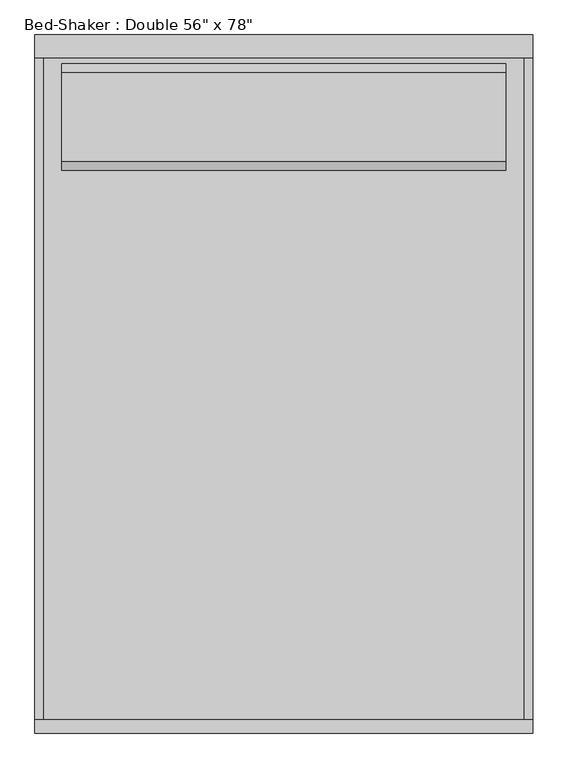
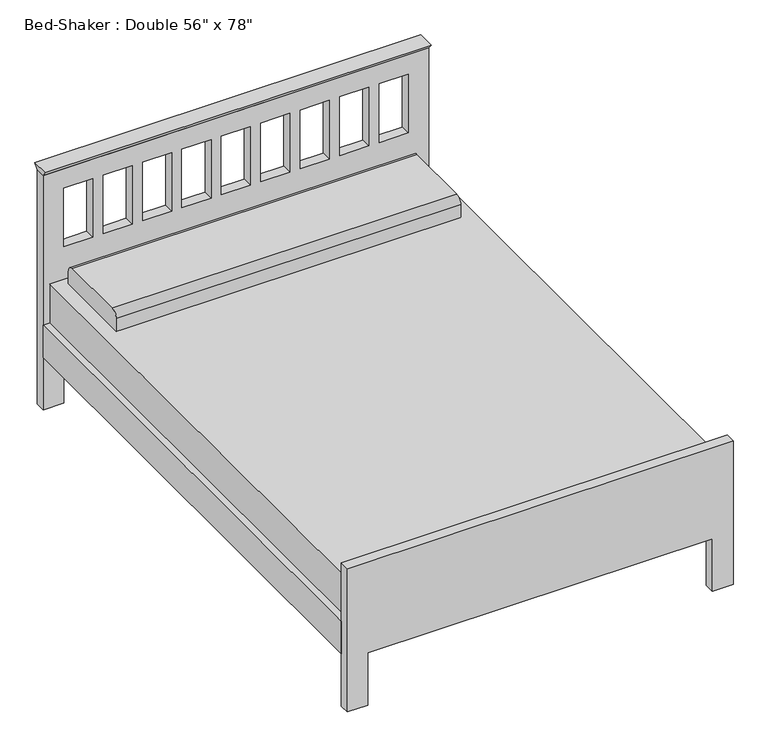
"""IFC4 building model written with IfcOpenShell, lengths in millimetres: furniture geometry."""

from ifc_helpers import new_model, si_unit, point, frame, frame_2d, origin, place, context, project, spatial, polyline, circle_curve, trimmed, segment, composite_curve, outline, extrude, source, transform, mapped, element, save


def furniture_096e7f55(model_context):
    return source(origin(), model_context, "Body", "SweptSolid", [
        extrude(outline(polyline([(-38.1, 914.4), (-51.9545455, 933.45), (13.8545455, 933.45), (0.0, 914.4), (-38.1, 914.4)])), frame((-730.0365546, 0.0, 0.0), z_axis=(1.0, 0.0, 0.0), x_axis=(0.0, 1.0, 0.0)), (0.0, 0.0, 1.0), 1422.4533613),
        extrude(outline(composite_curve([segment(polyline([(-373.2486637, 482.6), (-373.2486637, 533.4)]), True, "CONTINUOUS"), segment(trimmed(circle_curve(frame_2d((-347.8486637, 533.4)), 25.4), [point((-373.2486637, 533.4))], [point((-347.8486637, 558.8))], False, "CARTESIAN"), True, "CONTINUOUS"), segment(polyline([(-347.8486637, 558.8), (-93.8486637, 558.8)]), True, "CONTINUOUS"), segment(trimmed(circle_curve(frame_2d((-93.8486637, 533.4)), 25.4), [point((-93.8486637, 558.8))], [point((-68.4486637, 533.4))], False, "CARTESIAN"), True, "CONTINUOUS"), segment(polyline([(-68.4486637, 533.4), (-68.4486637, 482.6), (-373.2486637, 482.6)]), True, "CONTINUOUS")], self_intersect=False)), frame((-654.05, 0.0, 0.0), z_axis=(1.0, 0.0, 0.0), x_axis=(0.0, 1.0, 0.0)), (0.0, 0.0, 1.0), 1270.0),
        extrude(outline(polyline([(666.75, -38.1), (666.75, -1943.1), (-704.85, -1943.1), (-704.85, -38.1), (666.75, -38.1)])), frame((0.0, 0.0, 228.6), z_axis=(0.0, 0.0, 1.0), x_axis=(1.0, 0.0, 0.0)), (0.0, 0.0, 1.0), 254.0),
        extrude(outline(polyline([(666.75, -1943.1), (666.75, -38.1), (692.15, -38.1), (692.15, -1943.1), (666.75, -1943.1)])), frame((0.0, 0.0, 203.0994861), z_axis=(0.0, 0.0, 1.0), x_axis=(1.0, 0.0, 0.0)), (0.0, 0.0, 1.0), 127.0),
        extrude(outline(polyline([(-730.25, -1943.1), (-730.25, -38.1), (-704.85, -38.1), (-704.85, -1943.1), (-730.25, -1943.1)])), frame((0.0, 0.0, 203.5755296), z_axis=(0.0, 0.0, 1.0), x_axis=(1.0, 0.0, 0.0)), (0.0, 0.0, 1.0), 127.0),
        extrude(outline(polyline([(0.0, -654.05), (203.2, -654.05), (203.2, 615.95), (0.0, 615.95), (0.0, 692.15), (558.8, 692.15), (558.8, -730.25), (0.0, -730.25), (0.0, -654.05)])), frame((0.0, -1981.2, 0.0), z_axis=(0.0, 1.0, 0.0), x_axis=(0.0, 0.0, 1.0)), (0.0, 0.0, 1.0), 38.1),
        extrude(outline(polyline([(914.4, 692.4168067), (914.4, -730.0365546), (0.0, -730.0365546), (0.0, -654.05), (203.2, -654.05), (203.2, 615.95), (0.0, 615.95), (0.0, 692.4168067), (914.4, 692.4168067)]), holes=[polyline([(838.2, -546.8055556), (609.6, -546.8055556), (609.6, -654.05), (838.2, -654.05), (838.2, -546.8055556)]), polyline([(838.2, -401.4611111), (609.6, -401.4611111), (609.6, -508.7055556), (838.2, -508.7055556), (838.2, -401.4611111)]), polyline([(838.2, -256.1166667), (609.6, -256.1166667), (609.6, -363.3611111), (838.2, -363.3611111), (838.2, -256.1166667)]), polyline([(838.2, -110.7722222), (609.6, -110.7722222), (609.6, -218.0166667), (838.2, -218.0166667), (838.2, -110.7722222)]), polyline([(838.2, 179.9166667), (609.6, 179.9166667), (609.6, 72.6722222), (838.2, 72.6722222), (838.2, 179.9166667)]), polyline([(838.2, 325.2611111), (609.6, 325.2611111), (609.6, 218.0166667), (838.2, 218.0166667), (838.2, 325.2611111)]), polyline([(838.2, 470.6055556), (609.6, 470.6055556), (609.6, 363.3611111), (838.2, 363.3611111), (838.2, 470.6055556)]), polyline([(838.2, 615.95), (609.6, 615.95), (609.6, 508.7055556), (838.2, 508.7055556), (838.2, 615.95)]), polyline([(838.2, 34.5722222), (609.6, 34.5722222), (609.6, -72.6722222), (838.2, -72.6722222), (838.2, 34.5722222)])]), frame((0.0, -38.1, 0.0), z_axis=(0.0, 1.0, 0.0), x_axis=(0.0, 0.0, 1.0)), (0.0, 0.0, 1.0), 38.1),
    ])


if __name__ == "__main__":
    model = new_model("IFC4")
    model_context = context("Model", 3, world=origin())
    ifc_project = project(units=[si_unit("LENGTHUNIT", "METRE", prefix="MILLI")], contexts=[model_context])
    site = spatial("IfcSite", under=ifc_project)
    building = spatial("IfcBuilding", under=site)
    placement = place(None, origin())
    furniture_shape = furniture_096e7f55(model_context)
    element("IfcFurniture", 1, ObjectType="Bed-Shaker : Double 56\" x 78\"", at=placement, inside=building, context=model_context, shape_type="MappedRepresentation", body=[
        mapped(furniture_shape, transform((0.0, 0.0, 0.0), x_axis=(1.0, 0.0, 0.0), y_axis=(0.0, 1.0, 0.0), z_axis=(0.0, 0.0, 1.0))),
    ])
    save(model, "model.ifc")

# Revit data of these elements
# Type "Bed-Shaker : Double 56\" x 78\""
#   Assembly Code = "E2020200"
#   Length = 6' - 6"
#   Width = 4' - 8"
#   Frame Material = Birch
#   Mattress Material = Linen, White
# Element 1 (IfcFurniture, "Bed-Shaker : Double 56\" x 78\"")
#   Materials on its faces: "Birch", "Linen, White"
# Materials
#   "Birch": class "Wood", colour RGB 224 178 126, transparency 0, Description = "Betula Alleghaniensis", Cost = 0
#   "Linen, White": class "Textile", colour RGB 247 247 239, transparency 0, Description = "Linen, white", Cost = 0
